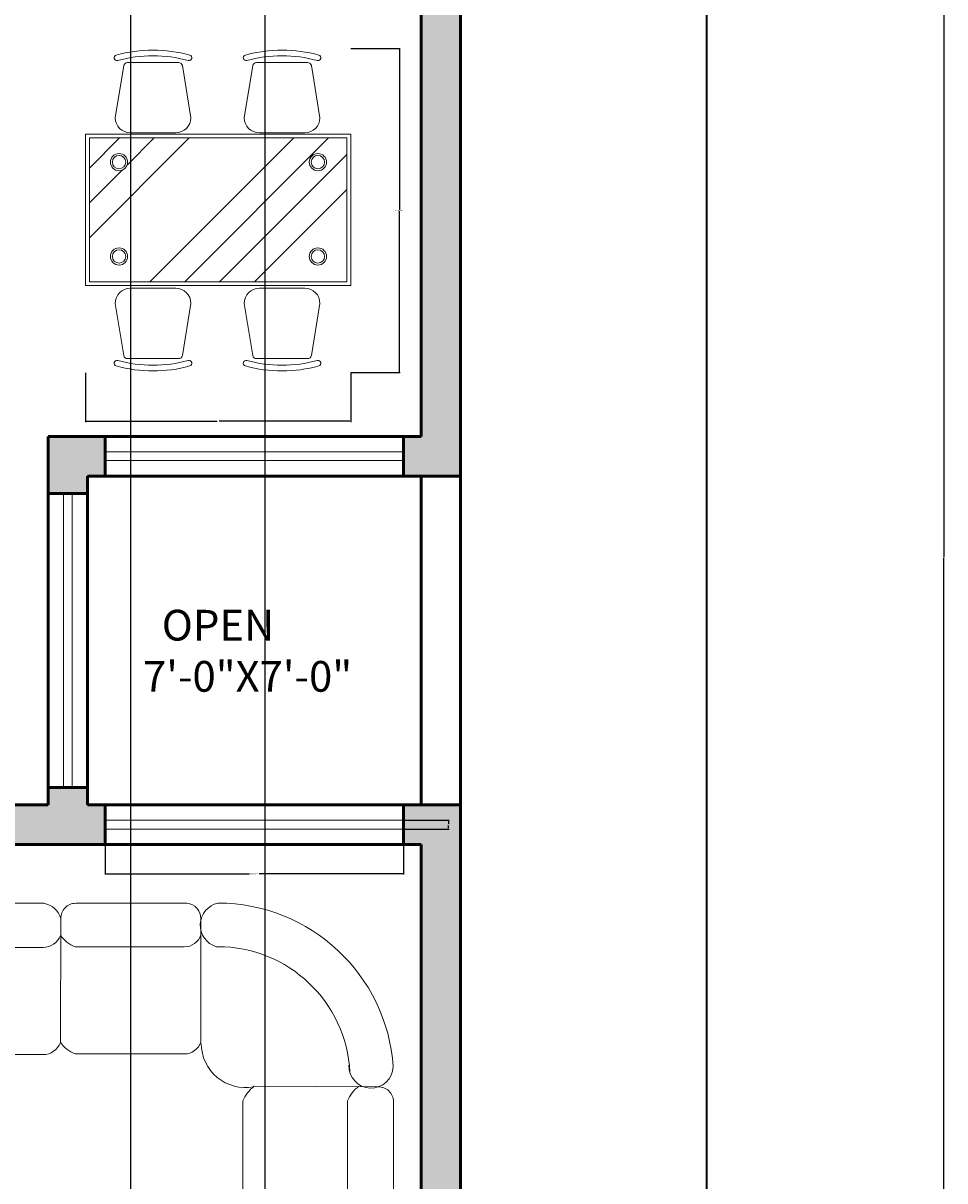
# Model space of a CAD drawing. Units: inches. Extents: x 2447 to 3157, y 2799 to 3988.
# Tile 7 of 9: x 2947 to 3157, y 3345 to 3609. Entities that reach past the tile are written whole.
import ezdxf

# ---------------------------------------------------------------- set-up
doc = ezdxf.new("R2010")
doc.units = ezdxf.units.IN
for name, color, linetype, lineweight in [('A-ANNO-DIMS', 2, 'Continuous', 18), ('A-AREA-IDEN', 7, 'Continuous', 25), ('A-FURN', 8, 'Continuous', 18), ('A-GLAZ', 4, 'Continuous', 18), ('A-WALL', 7, 'Continuous', 50), ('A-WALL-PATT', 252, 'Continuous', 13), ('C-PROP', 6, 'Continuous', 35)]:
    doc.layers.add(name, color=color, linetype=linetype, lineweight=lineweight)
doc.styles.get("Standard").update_dxf_attribs({"font": 'arial.ttf'})
doc.dimstyles.get("Standard").update_dxf_attribs({"dimtxt": 0.18, "dimasz": 0.18, "dimexe": 0.18, "dimexo": 0.0625, "dimgap": 0.09, "dimtad": 0, "dimtih": 1, "dimtoh": 1, "dimdec": 4, "dimzin": 0, "dimdsep": 46, "dimtxsty": 'Standard', "dimcen": 0.09, "dimadec": 0, "dimazin": 0, "dimtfac": 1, "dimtdec": 4, "dimtofl": 0, "dimtmove": 0, "dimatfit": 3, "dimfxl": 1, "dimtolj": 1, "dimtzin": 0, "dimarcsym": 0})

# ---------------------------------------------------------------- blocks, each defined once
blk = doc.blocks.new('A$C0FD55737')
for p, q in [((0.2013, 1.6134), (0.1562, 1.3384)), ((0.4912, 1.6302), (0.2211, 1.6302)), ((0.511, 1.6134), (0.5562, 1.3384)), ((0.8828, 1.6134), (0.8376, 1.3384)), ((0.9026, 1.6302), (1.1727, 1.6302)), ((1.1925, 1.6134), (1.2376, 1.3384)), ((0, 1.2513), (0, 0.4513)), ((1.4, 1.2513), (0, 1.2513)), ((0.02, 1.0725), (0.1788, 1.2313)), ((0.02, 0.7043), (0.547, 1.2313)), ((1.38, 1.2313), (0.02, 1.2313)), ((0.02, 1.2313), (0.02, 0.4713)), ((0.2189, 1.0873), (0.3629, 1.2313)), ((0.2362, 1.2584), (0.4762, 1.2584)), ((0.3393, 0.4713), (1.0993, 1.2313)), ((0.5234, 0.4713), (1.2834, 1.2313)), ((1.1576, 1.2584), (0.9176, 1.2584)), ((1.38, 0.4713), (1.38, 1.2313)), ((1.4, 0.4513), (1.4, 1.2513)), ((0.7074, 0.4713), (1.38, 1.1438)), ((0.02, 0.8884), (0.1931, 1.0614)), ((0.8915, 0.4713), (1.38, 0.9597)), ((0, 0.4513), (1.4, 0.4513)), ((0.02, 0.4713), (1.38, 0.4713)), ((0.2362, 0.4371), (0.4762, 0.4371)), ((1.1576, 0.4371), (0.9176, 0.4371)), ((0.2013, 0.0821), (0.1562, 0.3571)), ((0.511, 0.0821), (0.5562, 0.3571)), ((0.8828, 0.0821), (0.8376, 0.3571)), ((1.1925, 0.0821), (1.2376, 0.3571)), ((0.4912, 0.0653), (0.2211, 0.0653)), ((0.9026, 0.0653), (1.1727, 0.0653))]:
    blk.add_line(p, q)
for centre, radius in [((0.1766, 1.1037), 0.0454), ((0.1766, 1.1037), 0.0354), ((1.227, 1.1037), 0.0454), ((1.227, 1.1037), 0.0354), ((0.1766, 0.6052), 0.0454), ((0.1766, 0.6052), 0.0354), ((1.227, 0.6052), 0.0454), ((1.227, 0.6052), 0.0354)]:
    blk.add_circle(centre, radius)
for centre, radius, start, end in [((0.1662, 1.6546), 0.015, 105.49005, 284.28424), ((0.3562, 0.9712), 0.7243, 74.47014, 105.57697), ((0.3562, 0.9716), 0.6939, 74.43245, 105.56755), ((0.5461, 1.6546), 0.015, 255.71576, 74.50995), ((0.8477, 1.6546), 0.015, 105.49005, 284.28424), ((1.0376, 0.9712), 0.7243, 74.42303, 105.52986), ((1.0376, 0.9716), 0.6939, 74.43245, 105.56755), ((1.2276, 1.6546), 0.015, 255.71576, 74.50995), ((0.2211, 1.6102), 0.02, 90, 170.67171), ((0.4912, 1.6102), 0.02, 9.32829, 90), ((0.9026, 1.6102), 0.02, 90, 170.67171), ((1.1727, 1.6102), 0.02, 9.32829, 90), ((0.2362, 1.3384), 0.08, 180, 270), ((0.4762, 1.3384), 0.08, 270, 0), ((0.9176, 1.3384), 0.08, 180, 270), ((1.1576, 1.3384), 0.08, 270, 0), ((0.2362, 0.3571), 0.08, 90, 180), ((0.4762, 0.3571), 0.08, 0, 90), ((0.9176, 0.3571), 0.08, 90, 180), ((1.1576, 0.3571), 0.08, 0, 90), ((0.2211, 0.0853), 0.02, 189.32829, 270), ((0.4912, 0.0853), 0.02, 270, 350.67171), ((0.9026, 0.0853), 0.02, 189.32829, 270), ((1.1727, 0.0853), 0.02, 270, 350.67171), ((0.1662, 0.0409), 0.015, 75.71576, 254.50995), ((0.3562, 0.7243), 0.7243, 254.42303, 285.52986), ((0.3562, 0.7239), 0.6939, 254.43245, 285.56755), ((0.5461, 0.0409), 0.015, 285.49005, 104.28424), ((0.8477, 0.0409), 0.015, 75.71576, 254.50995), ((1.0376, 0.7243), 0.7243, 254.47014, 285.57697), ((1.0376, 0.7239), 0.6939, 254.43245, 285.56755), ((1.2276, 0.0409), 0.015, 285.49005, 104.28424)]:
    blk.add_arc(centre, radius, start, end)
blk = doc.blocks.new('A$C2F471D6A')
for p, q in [((2695.9, 2657.3), (2692.2, 1939.9)), ((1797.2, 841.3), (2182.6, 1242.6)), ((1797.2, 833.9), (2189.8, 1242.6)), ((1797.2, 826.4), (2197, 1242.6)), ((1797.2, 818.9), (2204.2, 1242.6)), ((1797.2, 848.8), (2175.4, 1242.6)), ((2161.4, 709.9), (2615.3, 1243.3)), ((2168.6, 709.9), (2622.5, 1243.3)), ((2175.8, 709.9), (2629.7, 1243.3)), ((2183, 709.9), (2636.9, 1243.3)), ((2190.2, 709.9), (2644.1, 1243.3)), ((2197.4, 709.9), (2651.3, 1243.3)), ((2755.3, 709.9), (2980.5, 1000.5)), ((2762.5, 709.9), (2981.1, 992)), ((2769.7, 709.9), (2981.1, 982.7)), ((2776.9, 709.9), (2981.1, 973.4)), ((2784.1, 709.9), (2981.1, 964.1)), ((807.3, 817.6), (89.9, 821.3))]:
    blk.add_line(p, q)
for points in [[(0, 1730, -0.393715), (947.4, 2744.8)], [(946.9, 2744.9, -1), (937.9, 2487, 1)], [(1060.8, 1939.9, 0.132391), (1145.9, 1873.4), (1778.5, 1873.4, 0.326313), (1874.7, 1943.6), (1874.7, 2657.3, 0.389129), (1793.3, 2746), (1149.6, 2746, 0.426582), (1064.5, 2657.3, 0.287811)], [(252.5, 1720.4), (252.5, 1729.1, -0.399385), (979.3, 2493.9)], [(1060.8, 2545.7, 0.132391), (1145.9, 2479.2), (1778.5, 2479.2, 0.287096), (1869.3, 2536)], [(1878.2, 2536, 0.331063), (1959.6, 2475.5), (2433.2, 2475.5)], [(2433.2, 2475.5), (2592.3, 2475.5, 0.316456), (2692.2, 2545.7, 0.132391), (2777.2, 2479.2), (3409.9, 2479.2, 0.287096), (3500.7, 2536)], [(812.9, 1633.4, 0.469502), (1063.7, 1935.5, -1.204519)], [(252.5, 1720.4, -0.77294), (0, 1730, -1)], [(257.4, 558.6), (257.4, 717.7, 0.316456), (187.2, 817.6, 0.132391), (253.7, 902.7), (253.7, 1535.3, 0.326313), (183.5, 1631.5), (180.9, 1631.5, 0.389129)], [(180.9, 0.4, 0.385191), (257.4, 85.1), (257.4, 558.6)]]:
    blk.add_lwpolyline(points, format="xyb")
for points in [[(2433.2, 1869.7), (2592.3, 1869.7, 0.316456), (2692.2, 1939.9, 0.132391), (2777.2, 1873.4), (3409.9, 1873.4, 0.326313), (3506.1, 1943.6), (3506.1, 2657.3, 0.389129), (3424.7, 2746), (2780.9, 2746, 0.426582), (2695.9, 2657.3, 0.287811), (2596, 2746), (1970.7, 2746, 0.366167), (1874.5, 2664.7), (1874.5, 1954.7, 0.414362), (1959.6, 1869.7)], [(877.5, 558.6), (877.5, 717.7, 0.316456), (807.3, 817.6, 0.132391), (873.8, 902.7), (873.8, 1535.3, 0.326313), (803.6, 1631.5), (89.9, 1631.5, 0.389129), (1.2, 1550.1), (1.2, 906.4, 0.426582), (89.9, 821.3, 0.287811), (1.2, 721.4), (1.2, 96.2, 0.366167), (82.5, 0), (792.5, 0, 0.414362), (877.5, 85.1)]]:
    blk.add_lwpolyline(points, format="xyb", close=True)
blk.add_lwpolyline([(1064.5, 2657.3), (1060.8, 1939.9)])
for points in [[(1742.1, 652.3), (1742.1, 1300.3), (3038.1, 1300.3), (3038.1, 652.3)], [(2981.1, 1185.5), (2920, 1185.5), (2920, 1242.6), (1860.2, 1242.6), (1860.2, 1185.5), (1797.2, 1185.5), (1797.2, 762.2), (1860.2, 762.2), (1860.2, 709.1), (2920, 709.1), (2920, 762.2), (2981.1, 762.2)]]:
    blk.add_lwpolyline(points, close=True)
blk = doc.blocks.new('GLAZING-68IN')
for p, q in [((0, 0), (68, 0)), ((0, -2), (68, -2))]:
    blk.add_line(p, q)
blk = doc.blocks.new('*D24')
at = {"layer": 'A-ANNO-DIMS', "color": 0, "lineweight": -2, "transparency": 16777216}
for p, q in [((2965.37, 3425.14), (2965.37, 3414.82)), ((3033.37, 3425.14), (3033.37, 3414.82)), ((2965.55, 3415), (2998.25, 3415)), ((3033.19, 3415), (3000.48, 3415))]:
    blk.add_line(p, q, dxfattribs=at)
at = {"layer": 'A-ANNO-DIMS', "color": 0, "transparency": 16777216}
for points in [[(2965.55, 3415.03), (2965.55, 3414.97), (2965.37, 3415)], [(3033.19, 3415.03), (3033.19, 3414.97), (3033.37, 3415)]]:
    blk.add_solid(points, dxfattribs=at)
at = {"layer": 'Defpoints', "color": 0, "transparency": 16777216}
for p in [(2965.37, 3425.2), (3033.37, 3425.2), (3033.37, 3415)]:
    blk.add_point(p, dxfattribs=at)
at = {"layer": 'A-ANNO-DIMS', "color": 0, "transparency": 16777216, "insert": (2999.37, 3415), "char_height": 0.18, "attachment_point": 5}
blk.add_mtext('\\A1;GLAZING 68 TYP.', dxfattribs=at)
blk = doc.blocks.new('*D25')
at = {"layer": 'A-ANNO-DIMS', "color": 0, "lineweight": -2, "transparency": 16777216}
for p, q in [((3033.43, 3427.2), (3043.75, 3427.2)), ((3043.57, 3427.02), (3043.57, 3426.38)), ((3033.43, 3425.2), (3043.75, 3425.2)), ((3043.57, 3425.38), (3043.57, 3426.02))]:
    blk.add_line(p, q, dxfattribs=at)
at = {"layer": 'A-ANNO-DIMS', "color": 0, "transparency": 16777216}
for points in [[(3043.54, 3427.02), (3043.6, 3427.02), (3043.57, 3427.2)], [(3043.54, 3425.38), (3043.6, 3425.38), (3043.57, 3425.2)]]:
    blk.add_solid(points, dxfattribs=at)
at = {"layer": 'Defpoints', "color": 0, "transparency": 16777216}
for p in [(3033.37, 3427.2), (3043.57, 3427.2), (3033.37, 3425.2)]:
    blk.add_point(p, dxfattribs=at)
at = {"layer": 'A-ANNO-DIMS', "color": 0, "transparency": 16777216, "insert": (3043.57, 3426.2), "char_height": 0.18, "attachment_point": 5}
blk.add_mtext('\\A1;2 TYP.', dxfattribs=at)
blk = doc.blocks.new('*D36')
at = {"layer": 'A-ANNO-DIMS', "color": 0, "lineweight": -2, "transparency": 16777216}
for p, q in [((3021.37, 3603.19), (3032.58, 3603.19)), ((3032.4, 3603.01), (3032.4, 3566.41)), ((3032.4, 3529.45), (3032.4, 3566.05)), ((3021.37, 3529.27), (3032.58, 3529.27))]:
    blk.add_line(p, q, dxfattribs=at)
at = {"layer": 'A-ANNO-DIMS', "color": 0, "transparency": 16777216}
for points in [[(3032.37, 3603.01), (3032.43, 3603.01), (3032.4, 3603.19)], [(3032.37, 3529.45), (3032.43, 3529.45), (3032.4, 3529.27)]]:
    blk.add_solid(points, dxfattribs=at)
at = {"layer": 'Defpoints', "color": 0, "transparency": 16777216}
for p in [(3021.31, 3603.19), (3032.4, 3603.19), (3021.31, 3529.27)]:
    blk.add_point(p, dxfattribs=at)
at = {"layer": 'A-ANNO-DIMS', "color": 0, "transparency": 16777216, "insert": (3032.4, 3566.23), "char_height": 0.18, "attachment_point": 5}
blk.add_mtext('\\A1;DINING SET 74', dxfattribs=at)
blk = doc.blocks.new('*D37')
at = {"layer": 'A-ANNO-DIMS', "color": 0, "lineweight": -2, "transparency": 16777216}
for p, q in [((2960.9, 3529.21), (2960.9, 3518)), ((3021.31, 3529.21), (3021.31, 3518)), ((2961.08, 3518.18), (2990.89, 3518.18)), ((3021.13, 3518.18), (2991.32, 3518.18))]:
    blk.add_line(p, q, dxfattribs=at)
at = {"layer": 'A-ANNO-DIMS', "color": 0, "transparency": 16777216}
for points in [[(2961.08, 3518.21), (2961.08, 3518.15), (2960.9, 3518.18)], [(3021.13, 3518.21), (3021.13, 3518.15), (3021.31, 3518.18)]]:
    blk.add_solid(points, dxfattribs=at)
at = {"layer": 'Defpoints', "color": 0, "transparency": 16777216}
for p in [(2960.9, 3529.27), (3021.31, 3529.27), (3021.31, 3518.18)]:
    blk.add_point(p, dxfattribs=at)
at = {"layer": 'A-ANNO-DIMS', "color": 0, "transparency": 16777216, "insert": (2991.11, 3518.18), "char_height": 0.18, "attachment_point": 5}
blk.add_mtext('\\A1;60', dxfattribs=at)
blk = doc.blocks.new('*D47')
at = {"layer": 'A-ANNO-DIMS', "color": 0, "lineweight": -2, "transparency": 16777216}
for p, q in [((2798.43, 3849.7), (3156.7, 3849.7)), ((3156.52, 3849.52), (3156.52, 3487.38)), ((3156.52, 3124.88), (3156.52, 3487.02)), ((3046.43, 3124.7), (3156.7, 3124.7))]:
    blk.add_line(p, q, dxfattribs=at)
at = {"layer": 'A-ANNO-DIMS', "color": 0, "transparency": 16777216}
for points in [[(3156.49, 3849.52), (3156.55, 3849.52), (3156.52, 3849.7)], [(3156.49, 3124.88), (3156.55, 3124.88), (3156.52, 3124.7)]]:
    blk.add_solid(points, dxfattribs=at)
at = {"layer": 'Defpoints', "color": 0, "transparency": 16777216}
for p in [(2798.37, 3849.7), (3156.52, 3849.7), (3046.37, 3124.7)]:
    blk.add_point(p, dxfattribs=at)
at = {"layer": 'A-ANNO-DIMS', "color": 0, "transparency": 16777216, "insert": (3156.52, 3487.2), "char_height": 0.18, "attachment_point": 5}
blk.add_mtext('\\A1;725', dxfattribs=at)
blk = doc.blocks.new('*D70')
at = {"layer": 'A-ANNO-DIMS', "color": 0, "lineweight": -2, "transparency": 16777216}
for p, q in [((3001.81, 2980.76), (3001.81, 3988.03)), ((3001.99, 3987.85), (3051.63, 3987.85)), ((3102.19, 3987.85), (3052.54, 3987.85)), ((3102.37, 2853.76), (3102.37, 3988.03))]:
    blk.add_line(p, q, dxfattribs=at)
at = {"layer": 'A-ANNO-DIMS', "color": 0, "transparency": 16777216}
for points in [[(3001.99, 3987.88), (3001.99, 3987.82), (3001.81, 3987.85)], [(3102.19, 3987.88), (3102.19, 3987.82), (3102.37, 3987.85)]]:
    blk.add_solid(points, dxfattribs=at)
at = {"layer": 'Defpoints', "color": 0, "transparency": 16777216}
for p in [(3102.37, 3987.85), (3001.81, 2980.7), (3102.37, 2853.7)]:
    blk.add_point(p, dxfattribs=at)
at = {"layer": 'A-ANNO-DIMS', "color": 0, "transparency": 16777216, "insert": (3052.09, 3987.85), "char_height": 0.18, "attachment_point": 5}
blk.add_mtext('\\A1;100.56', dxfattribs=at)
blk = doc.blocks.new('*D76')
at = {"layer": 'A-ANNO-DIMS', "color": 0, "lineweight": -2, "transparency": 16777216}
for p, q in [((2847.64, 3124.76), (2847.64, 3988.03)), ((2847.82, 3987.85), (2908.95, 3987.85)), ((2970.99, 3987.85), (2909.86, 3987.85)), ((2971.17, 3124.76), (2971.17, 3988.03))]:
    blk.add_line(p, q, dxfattribs=at)
at = {"layer": 'A-ANNO-DIMS', "color": 0, "transparency": 16777216}
for points in [[(2847.82, 3987.88), (2847.82, 3987.82), (2847.64, 3987.85)], [(2970.99, 3987.88), (2970.99, 3987.82), (2971.17, 3987.85)]]:
    blk.add_solid(points, dxfattribs=at)
at = {"layer": 'Defpoints', "color": 0, "transparency": 16777216}
for p in [(2971.17, 3987.85), (2847.64, 3124.7), (2971.17, 3124.7)]:
    blk.add_point(p, dxfattribs=at)
at = {"layer": 'A-ANNO-DIMS', "color": 0, "transparency": 16777216, "insert": (2909.4, 3987.85), "char_height": 0.18, "attachment_point": 5}
blk.add_mtext('\\A1;123.53', dxfattribs=at)

msp = doc.modelspace()

# ---------------------------------------------------------------- hatches: boundary and pattern name
at = {"layer": 'A-WALL-PATT'}
h = msp.add_hatch(color=256, dxfattribs=at)
h.dxf.hatch_style = 1
h.paths.add_polyline_path([(2570.3672, 3550.7002), (2726.3672, 3550.7002), (2726.3672, 3370.7002), (2722.3672, 3370.7002), (2722.3672, 3365.7002), (2739.3672, 3365.7002), (2739.3672, 3374.7002), (2735.3672, 3374.7002), (2735.3672, 3563.7002), (2726.3672, 3563.7002), (2726.3672, 3559.7002), (2570.3672, 3559.7002), (2570.3672, 3599.2479), (2561.3672, 3599.2479), (2561.3672, 3508.7002), (2570.3672, 3508.7002)])
h.paths.add_polyline_path([(2570.3672, 3412.7002), (2561.3672, 3412.7002), (2561.3672, 3331.9279), (2570.3672, 3331.9279), (2570.3672, 3365.7002), (2666.3672, 3365.7002), (2666.3672, 3361.7002), (2671.3672, 3361.7002), (2671.3672, 3365.7002), (2686.3672, 3365.7002), (2686.3672, 3370.7002), (2570.3672, 3370.7002)])
h.paths.add_polyline_path([(2965.3672, 3430.7002), (2961.3672, 3430.7002), (2961.3672, 3434.7002), (2952.3672, 3434.7002), (2952.3672, 3430.7002), (2847.6393, 3430.7002), (2812.3672, 3395.4282), (2812.3672, 3374.7002), (2781.3672, 3374.7002), (2781.3672, 3365.7002), (2812.3672, 3365.7002), (2812.3672, 3347.7002), (2821.3672, 3347.7002), (2821.3672, 3391.7002), (2851.3672, 3421.7002), (2965.3672, 3421.7002)])
h.paths.add_polyline_path([(3046.3672, 3430.7002), (3033.3672, 3430.7002), (3033.3672, 3421.7002), (3037.3672, 3421.7002), (3037.3672, 3133.7002), (2971.1661, 3133.7002), (2971.1661, 3124.7002), (3046.3672, 3124.7002)])
h.paths.add_polyline_path([(3046.3672, 3825.7002), (3005.5801, 3825.7002), (3005.5801, 3816.7002), (3037.3672, 3816.7002), (3037.3672, 3655.7002), (2940.3672, 3655.7002), (2940.3672, 3646.7002), (3037.3672, 3646.7002), (3037.3672, 3514.7002), (3033.3672, 3514.7002), (3033.3672, 3505.7002), (3046.3672, 3505.7002)])
h.paths.add_polyline_path([(2821.3672, 3258.7002), (2812.3672, 3258.7002), (2812.3672, 3240.7002), (2808.3672, 3240.7002), (2808.3672, 3231.7002), (2812.3672, 3231.7002), (2812.3672, 3223.0688), (2821.3672, 3223.0688)])
h.paths.add_polyline_path([(2766.3672, 3240.7002), (2707.3672, 3240.7002), (2707.3672, 3234.4466, -1), (2570.3672, 3234.4466), (2570.3672, 3240.5271), (2561.3672, 3240.5271), (2561.3672, 3234.4466, 0.98243292), (2716.3185, 3231.7002), (2766.3672, 3231.7002)])
h.paths.add_polyline_path([(2570.3672, 3307.9279), (2561.3672, 3307.9279), (2561.3672, 3281.7773), (2570.3672, 3281.7773), (2570.3672, 3284.7002), (2671.3672, 3284.7002), (2671.3672, 3331.7002), (2666.3672, 3331.7002), (2666.3672, 3293.7002), (2570.3672, 3293.7002)])
h.paths.add_polyline_path([(2570.3672, 3739.7002), (2574.3672, 3739.7002), (2574.3672, 3744.7002), (2570.3672, 3744.7002), (2570.3672, 3840.7002), (2614.3672, 3840.7002), (2614.3672, 3849.7002), (2561.3672, 3849.7002), (2561.3672, 3671.2479), (2570.3672, 3671.2479)])
h.paths.add_polyline_path([(2735.3672, 3840.7002), (2789.3672, 3840.7002), (2789.3672, 3816.7002), (2798.3672, 3816.7002), (2798.3672, 3849.7002), (2679.3672, 3849.7002), (2679.3672, 3840.7002), (2726.3672, 3840.7002), (2726.3672, 3778.7002), (2735.3672, 3778.7002)])
h.paths.add_polyline_path([(2651.3672, 3840.7002), (2655.3672, 3840.7002), (2655.3672, 3849.7002), (2638.3672, 3849.7002), (2638.3672, 3840.7002), (2642.3672, 3840.7002), (2642.3672, 3744.7002), (2610.3672, 3744.7002), (2610.3672, 3739.7002), (2726.3672, 3739.7002), (2726.3672, 3599.7002), (2735.3672, 3599.7002), (2735.3672, 3622.7002), (2739.3672, 3622.7002), (2739.3672, 3631.7002), (2735.3672, 3631.7002), (2735.3672, 3748.7002), (2726.3672, 3748.7002), (2726.3672, 3744.7002), (2651.3672, 3744.7002)])
h.paths.add_polyline_path([(2900.3672, 3816.7002), (2904.3672, 3816.7002), (2904.3672, 3825.7002), (2882.3672, 3825.7002), (2882.3672, 3816.7002), (2891.3672, 3816.7002), (2891.3672, 3650.4282), (2872.6393, 3631.7002), (2775.3672, 3631.7002), (2775.3672, 3622.7002), (2876.3672, 3622.7002), (2900.3672, 3646.7002), (2904.3672, 3646.7002), (2904.3672, 3655.7002), (2900.3672, 3655.7002)])
h.paths.add_polyline_path([(2957.5801, 3825.7002), (2940.3672, 3825.7002), (2940.3672, 3816.7002), (2957.5801, 3816.7002)], flags=17)
h = msp.add_hatch(color=256, dxfattribs=at)
h.dxf.hatch_style = 1
h.paths.add_polyline_path([(2965.3672, 3514.7002), (2952.3672, 3514.7002), (2952.3672, 3501.7002), (2961.3672, 3501.7002), (2961.3672, 3505.7002), (2965.3672, 3505.7002)])

# ---------------------------------------------------------------- linework, layer by layer
at = {"layer": 'A-GLAZ'}
for p, q in [((2955.8672, 3501.7002), (2955.8672, 3434.7002)), ((2957.8672, 3501.7002), (2957.8672, 3434.7002))]:
    msp.add_line(p, q, dxfattribs=at)
at = {"layer": 'A-WALL'}
for p, q in [((3046.3672, 3825.7002), (3046.3672, 3124.7002)), ((3037.3672, 3646.7002), (3037.3672, 3514.7002)), ((3037.3672, 3514.7002), (2952.3672, 3514.7002)), ((2952.3672, 3514.7002), (2952.3672, 3430.7002)), ((2965.3672, 3514.7002), (2965.3672, 3505.7002)), ((3033.3672, 3514.7002), (3033.3672, 3505.7002)), ((3046.3672, 3505.7002), (2961.3672, 3505.7002)), ((2961.3672, 3505.7002), (2961.3672, 3430.7002)), ((3037.3672, 3505.7002), (3037.3672, 3430.7002)), ((2961.3672, 3501.7002), (2952.3672, 3501.7002)), ((2961.3672, 3434.7002), (2952.3672, 3434.7002)), ((2952.3672, 3430.7002), (2847.6393, 3430.7002)), ((3046.3672, 3430.7002), (2961.3672, 3430.7002)), ((2965.3672, 3430.7002), (2965.3672, 3421.7002)), ((3033.3672, 3430.7002), (3033.3672, 3421.7002)), ((3037.3672, 3421.7002), (2851.3672, 3421.7002)), ((3037.3672, 3421.7002), (3037.3672, 3133.7002))]:
    msp.add_line(p, q, dxfattribs=at)
at = {"layer": 'C-PROP'}
msp.add_line((3102.3672, 3933.7002), (3102.3672, 2853.7002), dxfattribs=at)

# ---------------------------------------------------------------- block references
at = {"layer": 'A-FURN', "xscale": 43.14877990737321, "yscale": 43.14877990737321, "zscale": 43.14877990737321}
msp.add_blockref('A$C0FD55737', (2960.9013, 3529.6521), dxfattribs=at)
at = {"layer": 'A-FURN', "xscale": 0.0393700787401575, "yscale": 0.0393700787401575, "zscale": 0.0393700787401575, "rotation": 270}
msp.add_blockref('A$C2F471D6A', (2922.9523, 3408.3287), dxfattribs=at)
at = {"layer": 'A-GLAZ'}
for p in [(2965.3672, 3511.2002), (2965.3672, 3427.2002)]:
    msp.add_blockref('GLAZING-68IN', p, dxfattribs=at)

# ---------------------------------------------------------------- texts
at = {"layer": 'A-AREA-IDEN', "insert": (2973.9869, 3475.1906), "char_height": 7, "attachment_point": 1}
msp.add_mtext_dynamic_manual_height_columns('  OPEN\\P7\'-0"X7\'-0"', width=60.654222, gutter_width=12.5, heights=[0], dxfattribs=at)

# ---------------------------------------------------------------- dimensions: what is measured, and where the dimension line sits
at = {"layer": 'A-ANNO-DIMS'}
for base, p1, p2, override, picture, middle in [((2971.1661, 3987.8502), (2847.6393, 3124.7002), (2971.1661, 3124.7002), {"dimdec": 2, "dimlfac": 1, "dimrnd": 0, "dimzin": 0, "dimdsep": 46, "dimlunit": 2}, '*D76', (2909.4027, 3987.8502)), ((3102.3672, 3987.8502), (3001.807, 2980.7002), (3102.3672, 2853.7002), {"dimdec": 2, "dimlfac": 1, "dimrnd": 0, "dimzin": 0, "dimdsep": 46, "dimlunit": 2}, '*D70', (3052.0871, 3987.8502)), ((3021.3096, 3518.1808), (2960.9013, 3529.2695), (3021.3096, 3529.2695), {"dimdec": 0, "dimlfac": 1, "dimrnd": 0, "dimzin": 0, "dimdsep": 46, "dimlunit": 2}, '*D37', (2991.1054, 3518.1808))]:
    dim = msp.add_linear_dim(base=base, p1=p1, p2=p2, dimstyle='Standard', override=override, dxfattribs=at)
    dim.commit()
    dim.dimension.update_dxf_attribs({"geometry": picture, "text_midpoint": middle})
dim = msp.add_linear_dim(base=(3156.5172, 3849.7002), p1=(3046.3672, 3124.7002), p2=(2798.3672, 3849.7002), angle=90, dimstyle='Standard', override={"dimdec": 0, "dimlfac": 1, "dimrnd": 0, "dimzin": 0, "dimdsep": 46, "dimlunit": 2}, dxfattribs=at)
dim.commit()
dim.dimension.update_dxf_attribs({"geometry": '*D47', "text_midpoint": (3156.5172, 3487.2002)})
for base, p1, p2, text, picture, middle in [((3032.3983, 3603.1941), (3021.3096, 3529.2695), (3021.3096, 3603.1941), 'DINING SET <>', '*D36', (3032.3983, 3566.2318)), ((3043.5672, 3427.2002), (3033.3672, 3425.2002), (3033.3672, 3427.2002), '<> TYP.', '*D25', (3043.5672, 3426.2002))]:
    dim = msp.add_linear_dim(base=base, p1=p1, p2=p2, angle=90, text=text, dimstyle='Standard', override={"dimdec": 0, "dimlfac": 1, "dimrnd": 0, "dimzin": 0, "dimdsep": 46, "dimlunit": 2}, dxfattribs=at)
    dim.commit()
    dim.dimension.update_dxf_attribs({"geometry": picture, "text_midpoint": middle})
dim = msp.add_linear_dim(base=(3033.3672, 3415.0002), p1=(2965.3672, 3425.2002), p2=(3033.3672, 3425.2002), text='GLAZING <> TYP.', dimstyle='Standard', override={"dimdec": 0, "dimlfac": 1, "dimrnd": 0, "dimzin": 0, "dimdsep": 46, "dimlunit": 2}, dxfattribs=at)
dim.commit()
dim.dimension.update_dxf_attribs({"geometry": '*D24', "text_midpoint": (2999.3672, 3415.0002)})

doc.saveas('drawing.dxf')
